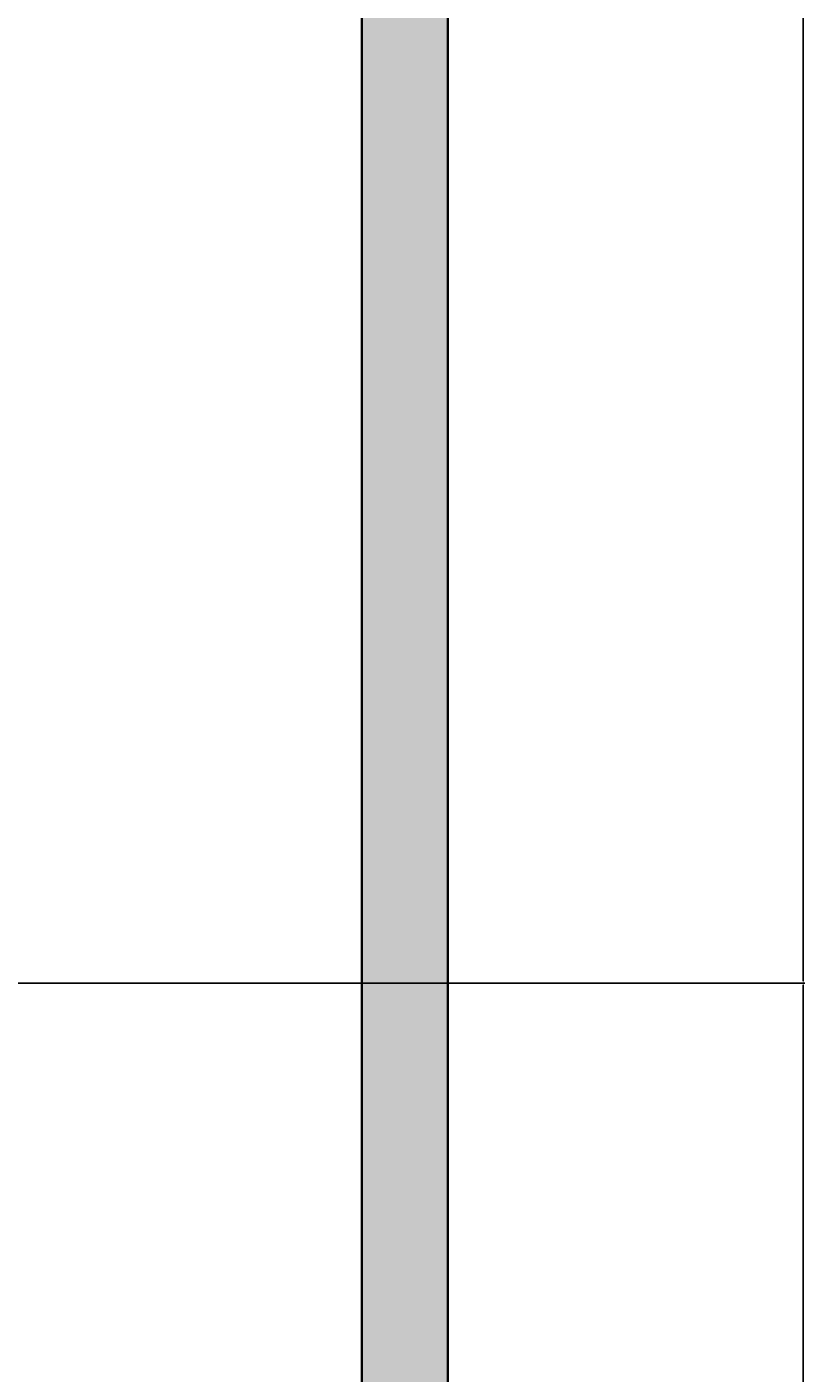
# Model space of a CAD drawing. Units: inches. Extents: x 2701 to 6846, y 811 to 2447.
# Tile 6 of 20: x 3102 to 3183, y 989 to 1130. Entities that reach past the tile are written whole.
import ezdxf

# ---------------------------------------------------------------- set-up
doc = ezdxf.new("R2010")
doc.units = ezdxf.units.IN
doc.layers.add('A-ANNO-DIMS', color=2, linetype='Continuous', lineweight=18)
doc.layers.add('C-PROP', color=7, linetype='Continuous', lineweight=35)
doc.layers.add('C-PROP-PATT', color=18, linetype='Continuous', lineweight=13, true_color=0x000000)
doc.styles.get("Standard").update_dxf_attribs({"font": 'arial.ttf'})
doc.dimstyles.get("Standard").update_dxf_attribs({"dimtxt": 0.18, "dimasz": 0.18, "dimexe": 0.18, "dimexo": 0.0625, "dimgap": 0.09, "dimtad": 0, "dimtih": 1, "dimtoh": 1, "dimdec": 4, "dimzin": 0, "dimdsep": 46, "dimtxsty": 'Standard', "dimcen": 0.09, "dimadec": 0, "dimazin": 0, "dimtfac": 1, "dimtdec": 4, "dimtofl": 0, "dimtmove": 0, "dimatfit": 3, "dimfxl": 1, "dimtolj": 1, "dimtzin": 0, "dimarcsym": 0})

# ---------------------------------------------------------------- blocks, each defined once
blk = doc.blocks.new('*D68')
at = {"layer": 'A-ANNO-DIMS', "color": 0, "lineweight": -2, "transparency": 16777216}
for p, q in [((3092.03, 1462.05), (3183.35, 1462.05)), ((3183.17, 1461.87), (3183.17, 1246.23)), ((3183.17, 1030.23), (3183.17, 1245.87)), ((3092.03, 1030.05), (3183.35, 1030.05))]:
    blk.add_line(p, q, dxfattribs=at)
at = {"layer": 'A-ANNO-DIMS', "color": 0, "transparency": 16777216}
for points in [[(3183.14, 1461.87), (3183.2, 1461.87), (3183.17, 1462.05)], [(3183.14, 1030.23), (3183.2, 1030.23), (3183.17, 1030.05)]]:
    blk.add_solid(points, dxfattribs=at)
at = {"layer": 'Defpoints', "color": 0, "transparency": 16777216}
for p in [(3091.97, 1462.05), (3183.17, 1462.05), (3091.97, 1030.05)]:
    blk.add_point(p, dxfattribs=at)
at = {"layer": 'A-ANNO-DIMS', "color": 0, "transparency": 16777216, "insert": (3183.17, 1246.05), "char_height": 0.18, "attachment_point": 5}
blk.add_mtext('\\A1;432', dxfattribs=at)
blk = doc.blocks.new('*D70')
at = {"layer": 'A-ANNO-DIMS', "color": 0, "lineweight": -2, "transparency": 16777216}
for p, q in [((3092.03, 1030.05), (3183.35, 1030.05)), ((3183.17, 1029.87), (3183.17, 943.23)), ((3183.17, 856.23), (3183.17, 942.87)), ((3146.03, 856.05), (3183.35, 856.05))]:
    blk.add_line(p, q, dxfattribs=at)
at = {"layer": 'A-ANNO-DIMS', "color": 0, "transparency": 16777216}
for points in [[(3183.14, 1029.87), (3183.2, 1029.87), (3183.17, 1030.05)], [(3183.14, 856.23), (3183.2, 856.23), (3183.17, 856.05)]]:
    blk.add_solid(points, dxfattribs=at)
at = {"layer": 'Defpoints', "color": 0, "transparency": 16777216}
for p in [(3091.97, 1030.05), (3183.17, 1030.05), (3145.97, 856.05)]:
    blk.add_point(p, dxfattribs=at)
at = {"layer": 'A-ANNO-DIMS', "color": 0, "transparency": 16777216, "insert": (3183.17, 943.05), "char_height": 0.18, "attachment_point": 5}
blk.add_mtext('\\A1;174', dxfattribs=at)

msp = doc.modelspace()

# ---------------------------------------------------------------- hatches: boundary and pattern name
at = {"layer": 'C-PROP-PATT'}
h = msp.add_hatch(color=256, dxfattribs=at)
h.dxf.hatch_style = 1
h.paths.add_polyline_path([(3145.97, 1504.05), (2737.97, 1504.05), (2737.97, 967.05), (2746.97, 967.05), (2746.97, 1495.05), (3136.97, 1495.05), (3136.97, 865.05), (3130.97, 865.05), (3130.97, 856.05), (3145.97, 856.05)])
h.paths.add_polyline_path([(3070.97, 865.05), (2746.97, 865.05), (2746.97, 871.05), (2737.97, 871.05), (2737.97, 856.05), (3070.97, 856.05)], flags=17)

# ---------------------------------------------------------------- linework, layer by layer
at = {"layer": 'C-PROP'}
for p, q in [((3145.97, 1504.05), (3145.97, 856.05)), ((3136.97, 1495.05), (3136.97, 865.05))]:
    msp.add_line(p, q, dxfattribs=at)

# ---------------------------------------------------------------- dimensions: what is measured, and where the dimension line sits
at = {"layer": 'A-ANNO-DIMS'}
for base, p1, p2, picture, middle in [((3183.17, 1462.05), (3091.97, 1030.05), (3091.97, 1462.05), '*D68', (3183.17, 1246.05)), ((3183.17, 1030.05), (3145.97, 856.05), (3091.97, 1030.05), '*D70', (3183.17, 943.05))]:
    dim = msp.add_linear_dim(base=base, p1=p1, p2=p2, angle=90, dimstyle='Standard', override={"dimdec": 0, "dimlfac": 1, "dimrnd": 0, "dimzin": 0, "dimdsep": 46, "dimlunit": 2}, dxfattribs=at)
    dim.commit()
    dim.dimension.update_dxf_attribs({"geometry": picture, "text_midpoint": middle})

doc.saveas('drawing.dxf')
